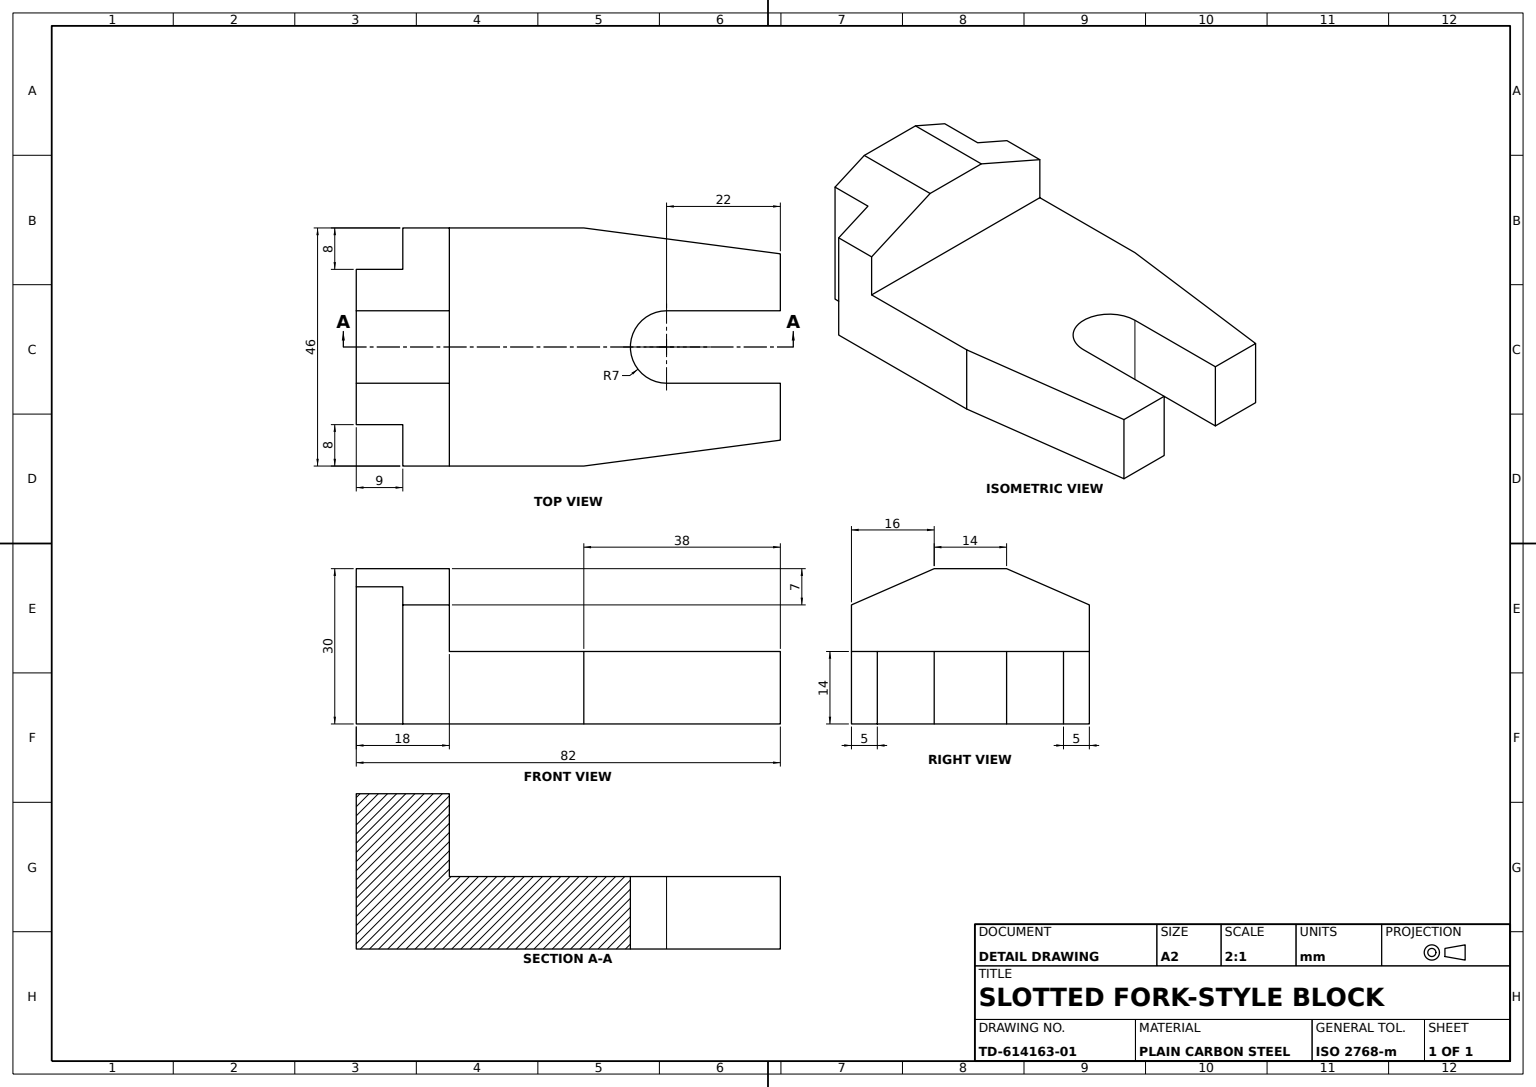
from build123d import *

# Parameters (mm, degrees)
SLOTTED_BASE_PLATE_DEPTH = 14
UPRIGHT_BLOCK_DEPTH      = 9
TOP_STEP_BOSS_DEPTH      = 9


with BuildPart() as part:
    # Base Plate Profile Sketch → Slotted Base Plate (new body)
    with BuildSketch(Plane(origin=(0, 0, 0), x_dir=(1, 0, 0), z_dir=(0, 1, 0))):
        Polygon((-22, -15), (-13, -15), (-13, -23), (22, -23), (22, 23), (-13, 23), (-13, 15), (-22, 15), align=None)
        with BuildLine():
            ThreePointArc((38, 7), (31, 0), (38, -7))
            Line((38, -7), (60, -7))
            Line((60, -7), (60, -18))
            Line((60, -18), (22, -23))
            Line((22, -23), (22, 23))
            Line((22, 23), (60, 18))
            Line((60, 18), (60, 7))
            Line((60, 7), (38, 7))
        make_face()
    extrude(amount=SLOTTED_BASE_PLATE_DEPTH)

    # Upright Block Sketch → Upright Block (add)
    with BuildSketch(Plane.ZY.offset(22)):
        Polygon((7, 30), (-7, 30), (-15, 26.5), (-15, 0), (15, 0), (15, 26.5), align=None)
    extrude(amount=-UPRIGHT_BLOCK_DEPTH)

    # Top Step Sketch → Top Step Boss (add)
    with BuildSketch(Plane.ZY.offset(13)):
        Polygon((-7, 30), (7, 30), (23, 23), (23, 0), (-23, 0), (-23, 23), align=None)
    extrude(amount=-TOP_STEP_BOSS_DEPTH)


solid = part.part
